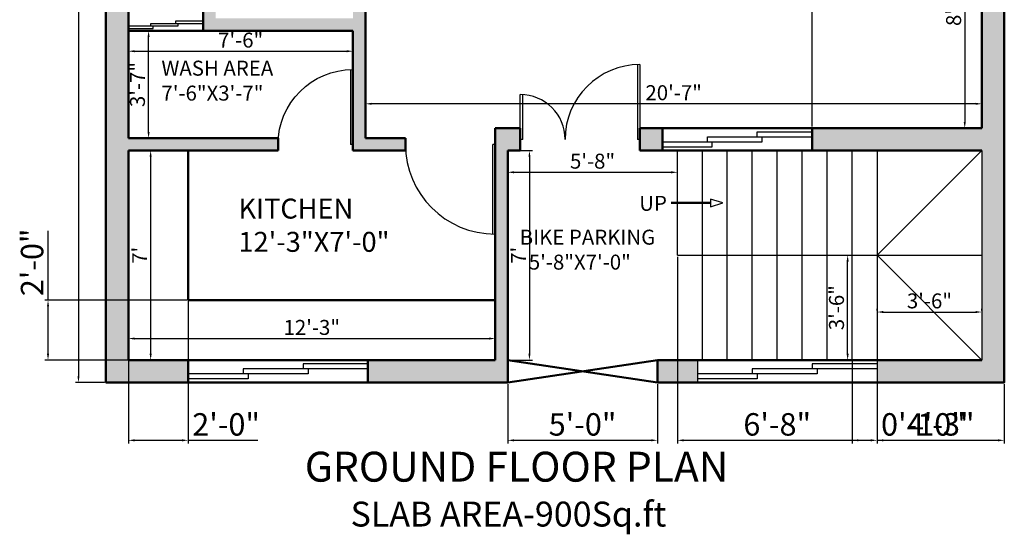
# Model space of a CAD drawing. Units: inches. Extents: x 3274 to 5176, y 1085 to 2172.
# Tile 1 of 16: x 3339 to 3733, y 1118 to 1325. Entities that reach past the tile are written whole.
import ezdxf

# ---------------------------------------------------------------- set-up
doc = ezdxf.new("R2010")
doc.units = ezdxf.units.IN
for name, color, linetype, lineweight in [('A-ANNO-DIMS', 2, 'Continuous', 18), ('A-ANNO-TEXT', 7, 'Continuous', 25), ('A-AREA-IDEN', 3, 'Continuous', 25), ('A-DOOR', 4, 'Continuous', 25), ('A-FLOR-STRS', 7, 'Continuous', 25), ('A-GLAZ', 5, 'Continuous', 25), ('A-WALL', 7, 'Continuous', 50), ('A-WALL-PATT', 8, 'Continuous', 13)]:
    doc.layers.add(name, color=color, linetype=linetype, lineweight=lineweight)
doc.styles.get("Standard").update_dxf_attribs({"font": 'arial.ttf'})
doc.dimstyles.new('ISO-25', dxfattribs={"dimtxt": 9, "dimasz": 2.5, "dimexe": 1.25, "dimexo": 0.625, "dimtad": 1, "dimdec": 1, "dimlunit": 3, "dimtxsty": 'Standard', "dimcen": 2.5, "dimclrd": 4, "dimclre": 4, "dimclrt": 1, "dimadec": 0, "dimazin": 0, "dimtfac": 1, "dimtdec": 1, "dimtmove": 0, "dimatfit": 3, "dimfxl": 1, "dimarcsym": 0})

# ---------------------------------------------------------------- blocks, each defined once
blk = doc.blocks.new('3')
for p, q in [((47, 30), (47, 0)), ((48, 30), (48, 0)), ((0, 0), (0, 18)), ((1, 0), (1, 18)), ((1, 0), (0, 0)), ((48, 0), (47, 0))]:
    blk.add_line(p, q)
for centre, radius, start, end in [((48, 0), 30, 90, 180), ((0, 0), 18, 0, 90)]:
    blk.add_arc(centre, radius, start, end)
blk = doc.blocks.new('2')
for p, q in [((0, 30), (0, 0)), ((1, 30), (1, 0)), ((0, 0), (1, 0))]:
    blk.add_line(p, q)
blk.add_arc((0, 0), 30, 0, 90)
blk = doc.blocks.new('1')
for p, q in [((0, 36), (0, 0)), ((1, 36), (1, 0)), ((0, 0), (1, 0))]:
    blk.add_line(p, q)
blk.add_arc((0, 0), 36, 0, 90)
blk = doc.blocks.new('*D11')
at = {"layer": 'A-ANNO-DIMS', "color": 0, "lineweight": -2, "transparency": 16777216}
for p, q in [((3372.68, 1539.28), (3361.05, 1539.28)), ((3362.3, 1536.78), (3362.3, 1181.78)), ((3372.68, 1179.28), (3361.05, 1179.28))]:
    blk.add_line(p, q, dxfattribs=at)
at = {"layer": 'A-ANNO-DIMS', "color": 0, "transparency": 16777216}
for points in [[(3361.88, 1536.78), (3362.71, 1536.78), (3362.3, 1539.28)], [(3361.88, 1181.78), (3362.71, 1181.78), (3362.3, 1179.28)]]:
    blk.add_solid(points, dxfattribs=at)
at = {"layer": 'Defpoints', "color": 0, "transparency": 16777216}
for p in [(3373.3, 1539.28), (3362.3, 1179.28), (3373.3, 1179.28)]:
    blk.add_point(p, dxfattribs=at)
at = {"layer": 'A-ANNO-DIMS', "color": 0, "transparency": 16777216, "insert": (3357.07, 1359.28), "char_height": 9, "attachment_point": 5, "rotation": 90}
blk.add_mtext("30'", dxfattribs=at)
blk = doc.blocks.new('*D20')
at = {"layer": 'A-ANNO-DIMS', "color": 0, "lineweight": -2, "transparency": 16777216}
for p, q in [((3382.93, 1320.28), (3391.65, 1320.28)), ((3390.4, 1279.78), (3390.4, 1317.78)), ((3382.93, 1277.28), (3391.65, 1277.28))]:
    blk.add_line(p, q, dxfattribs=at)
at = {"layer": 'A-ANNO-DIMS', "color": 0, "transparency": 16777216}
for points in [[(3389.98, 1317.78), (3390.82, 1317.78), (3390.4, 1320.28)], [(3389.98, 1279.78), (3390.82, 1279.78), (3390.4, 1277.28)]]:
    blk.add_solid(points, dxfattribs=at)
at = {"layer": 'Defpoints', "color": 0, "transparency": 16777216}
for p in [(3382.3, 1320.28), (3390.4, 1320.28), (3382.3, 1277.28)]:
    blk.add_point(p, dxfattribs=at)
at = {"layer": 'A-ANNO-DIMS', "color": 0, "transparency": 16777216, "insert": (3386.71, 1298.78), "char_height": 6, "attachment_point": 5, "rotation": 90}
blk.add_mtext('3\'-7"', dxfattribs=at)
blk = doc.blocks.new('*D21')
at = {"layer": 'A-ANNO-DIMS', "color": 0, "lineweight": -2, "transparency": 16777216}
for p, q in [((3382.3, 1319.66), (3382.3, 1310.87)), ((3472.3, 1319.66), (3472.3, 1310.87)), ((3384.8, 1312.12), (3469.8, 1312.12))]:
    blk.add_line(p, q, dxfattribs=at)
at = {"layer": 'A-ANNO-DIMS', "color": 0, "transparency": 16777216}
for points in [[(3384.8, 1312.54), (3384.8, 1311.7), (3382.3, 1312.12)], [(3469.8, 1312.54), (3469.8, 1311.7), (3472.3, 1312.12)]]:
    blk.add_solid(points, dxfattribs=at)
at = {"layer": 'Defpoints', "color": 0, "transparency": 16777216}
for p in [(3382.3, 1320.28), (3472.3, 1320.28), (3472.3, 1312.12)]:
    blk.add_point(p, dxfattribs=at)
at = {"layer": 'A-ANNO-DIMS', "color": 0, "transparency": 16777216, "insert": (3427.3, 1315.81), "char_height": 6, "attachment_point": 5}
blk.add_mtext('7\'-6"', dxfattribs=at)
blk = doc.blocks.new('*D22')
at = {"layer": 'A-ANNO-DIMS', "color": 0, "lineweight": -2, "transparency": 16777216}
for p, q in [((3382.93, 1272.28), (3392.47, 1272.28)), ((3391.22, 1269.78), (3391.22, 1190.78)), ((3382.93, 1188.28), (3392.47, 1188.28))]:
    blk.add_line(p, q, dxfattribs=at)
at = {"layer": 'A-ANNO-DIMS', "color": 0, "transparency": 16777216}
for points in [[(3390.81, 1269.78), (3391.64, 1269.78), (3391.22, 1272.28)], [(3390.81, 1190.78), (3391.64, 1190.78), (3391.22, 1188.28)]]:
    blk.add_solid(points, dxfattribs=at)
at = {"layer": 'Defpoints', "color": 0, "transparency": 16777216}
for p in [(3382.3, 1272.28), (3382.3, 1188.28), (3391.22, 1188.28)]:
    blk.add_point(p, dxfattribs=at)
at = {"layer": 'A-ANNO-DIMS', "color": 0, "transparency": 16777216, "insert": (3387.6, 1230.28), "char_height": 6, "attachment_point": 5, "rotation": 90}
blk.add_mtext("7'", dxfattribs=at)
blk = doc.blocks.new('*D23')
at = {"layer": 'A-ANNO-DIMS', "color": 0, "lineweight": -2, "transparency": 16777216}
for p, q in [((3382.3, 1188.91), (3382.3, 1198.14)), ((3384.8, 1196.89), (3526.8, 1196.89)), ((3529.3, 1188.91), (3529.3, 1198.14))]:
    blk.add_line(p, q, dxfattribs=at)
at = {"layer": 'A-ANNO-DIMS', "color": 0, "transparency": 16777216}
for points in [[(3384.8, 1197.31), (3384.8, 1196.47), (3382.3, 1196.89)], [(3526.8, 1197.31), (3526.8, 1196.47), (3529.3, 1196.89)]]:
    blk.add_solid(points, dxfattribs=at)
at = {"layer": 'Defpoints', "color": 0, "transparency": 16777216}
for p in [(3529.3, 1196.89), (3382.3, 1188.28), (3529.3, 1188.28)]:
    blk.add_point(p, dxfattribs=at)
at = {"layer": 'A-ANNO-DIMS', "color": 0, "transparency": 16777216, "insert": (3455.8, 1200.58), "char_height": 6, "attachment_point": 5}
blk.add_mtext('12\'-3"', dxfattribs=at)
blk = doc.blocks.new('*D24')
at = {"layer": 'A-ANNO-DIMS', "color": 0, "lineweight": -2, "transparency": 16777216}
for p, q in [((3534.3, 1262.94), (3534.3, 1262.32)), ((3536.8, 1263.57), (3599.8, 1263.57)), ((3602.3, 1264.19), (3602.3, 1264.82))]:
    blk.add_line(p, q, dxfattribs=at)
at = {"layer": 'A-ANNO-DIMS', "color": 0, "transparency": 16777216}
for points in [[(3536.8, 1263.99), (3536.8, 1263.15), (3534.3, 1263.57)], [(3599.8, 1263.99), (3599.8, 1263.15), (3602.3, 1263.57)]]:
    blk.add_solid(points, dxfattribs=at)
at = {"layer": 'Defpoints', "color": 0, "transparency": 16777216}
for p in [(3534.3, 1263.57), (3602.3, 1263.57), (3602.3, 1263.57)]:
    blk.add_point(p, dxfattribs=at)
at = {"layer": 'A-ANNO-DIMS', "color": 0, "transparency": 16777216, "insert": (3568.3, 1267.26), "char_height": 6, "attachment_point": 5}
blk.add_mtext('5\'-8"', dxfattribs=at)
blk = doc.blocks.new('*D25')
at = {"layer": 'A-ANNO-DIMS', "color": 0, "lineweight": -2, "transparency": 16777216}
for p, q in [((3534.93, 1272.28), (3544.26, 1272.28)), ((3543.01, 1269.78), (3543.01, 1190.78)), ((3534.93, 1188.28), (3544.26, 1188.28))]:
    blk.add_line(p, q, dxfattribs=at)
at = {"layer": 'A-ANNO-DIMS', "color": 0, "transparency": 16777216}
for points in [[(3542.6, 1269.78), (3543.43, 1269.78), (3543.01, 1272.28)], [(3542.6, 1190.78), (3543.43, 1190.78), (3543.01, 1188.28)]]:
    blk.add_solid(points, dxfattribs=at)
at = {"layer": 'Defpoints', "color": 0, "transparency": 16777216}
for p in [(3534.3, 1272.28), (3534.3, 1188.28), (3543.01, 1188.28)]:
    blk.add_point(p, dxfattribs=at)
at = {"layer": 'A-ANNO-DIMS', "color": 0, "transparency": 16777216, "insert": (3539.39, 1230.28), "char_height": 6, "attachment_point": 5, "rotation": 90}
blk.add_mtext("7'", dxfattribs=at)
blk = doc.blocks.new('*D26')
at = {"layer": 'A-ANNO-DIMS', "color": 0, "lineweight": -2, "transparency": 16777216}
for p, q in [((3668.38, 1230.28), (3671.77, 1230.28)), ((3670.52, 1190.78), (3670.52, 1227.78)), ((3668.38, 1188.28), (3671.77, 1188.28))]:
    blk.add_line(p, q, dxfattribs=at)
at = {"layer": 'A-ANNO-DIMS', "color": 0, "transparency": 16777216}
for points in [[(3670.1, 1227.78), (3670.94, 1227.78), (3670.52, 1230.28)], [(3670.1, 1190.78), (3670.94, 1190.78), (3670.52, 1188.28)]]:
    blk.add_solid(points, dxfattribs=at)
at = {"layer": 'Defpoints', "color": 0, "transparency": 16777216}
for p in [(3667.75, 1230.28), (3670.52, 1230.28), (3667.75, 1188.28)]:
    blk.add_point(p, dxfattribs=at)
at = {"layer": 'A-ANNO-DIMS', "color": 0, "transparency": 16777216, "insert": (3666.83, 1209.28), "char_height": 6, "attachment_point": 5, "rotation": 90}
blk.add_mtext('3\'-6"', dxfattribs=at)
blk = doc.blocks.new('*D27')
at = {"layer": 'A-ANNO-DIMS', "color": 0, "lineweight": -2, "transparency": 16777216}
for p, q in [((3682.3, 1208.15), (3682.3, 1208.78)), ((3684.8, 1207.53), (3721.8, 1207.53)), ((3724.3, 1208.15), (3724.3, 1208.78))]:
    blk.add_line(p, q, dxfattribs=at)
at = {"layer": 'A-ANNO-DIMS', "color": 0, "transparency": 16777216}
for points in [[(3684.8, 1207.95), (3684.8, 1207.11), (3682.3, 1207.53)], [(3721.8, 1207.95), (3721.8, 1207.11), (3724.3, 1207.53)]]:
    blk.add_solid(points, dxfattribs=at)
at = {"layer": 'Defpoints', "color": 0, "transparency": 16777216}
for p in [(3682.3, 1207.53), (3724.3, 1207.53), (3724.3, 1207.53)]:
    blk.add_point(p, dxfattribs=at)
at = {"layer": 'A-ANNO-DIMS', "color": 0, "transparency": 16777216, "insert": (3703.3, 1211.22), "char_height": 6, "attachment_point": 5}
blk.add_mtext('3\'-6"', dxfattribs=at)
blk = doc.blocks.new('*D28')
at = {"layer": 'A-ANNO-DIMS', "color": 0, "lineweight": -2, "transparency": 16777216}
for p, q in [((3723.68, 1381.28), (3716.2, 1381.28)), ((3717.45, 1378.78), (3717.45, 1283.78)), ((3723.68, 1281.28), (3716.2, 1281.28))]:
    blk.add_line(p, q, dxfattribs=at)
at = {"layer": 'A-ANNO-DIMS', "color": 0, "transparency": 16777216}
for points in [[(3717.03, 1378.78), (3717.86, 1378.78), (3717.45, 1381.28)], [(3717.03, 1283.78), (3717.86, 1283.78), (3717.45, 1281.28)]]:
    blk.add_solid(points, dxfattribs=at)
at = {"layer": 'Defpoints', "color": 0, "transparency": 16777216}
for p in [(3724.3, 1381.28), (3717.45, 1281.28), (3724.3, 1281.28)]:
    blk.add_point(p, dxfattribs=at)
at = {"layer": 'A-ANNO-DIMS', "color": 0, "transparency": 16777216, "insert": (3713.76, 1331.28), "char_height": 6, "attachment_point": 5, "rotation": 90}
blk.add_mtext('8\'-4"', dxfattribs=at)
blk = doc.blocks.new('*D29')
at = {"layer": 'A-ANNO-DIMS', "color": 0, "lineweight": -2, "transparency": 16777216}
for p, q in [((3477.3, 1277.91), (3477.3, 1292.29)), ((3721.8, 1291.04), (3479.8, 1291.04)), ((3724.3, 1281.91), (3724.3, 1292.29))]:
    blk.add_line(p, q, dxfattribs=at)
at = {"layer": 'A-ANNO-DIMS', "color": 0, "transparency": 16777216}
for points in [[(3479.8, 1291.45), (3479.8, 1290.62), (3477.3, 1291.04)], [(3721.8, 1291.45), (3721.8, 1290.62), (3724.3, 1291.04)]]:
    blk.add_solid(points, dxfattribs=at)
at = {"layer": 'Defpoints', "color": 0, "transparency": 16777216}
for p in [(3477.3, 1291.04), (3724.3, 1281.28), (3477.3, 1277.28)]:
    blk.add_point(p, dxfattribs=at)
at = {"layer": 'A-ANNO-DIMS', "color": 0, "transparency": 16777216, "insert": (3600.8, 1294.72), "char_height": 6, "attachment_point": 5}
blk.add_mtext('20\'-7"', dxfattribs=at)
blk = doc.blocks.new('WIN-30')
for p, q in [((4385.19, 1318.35), (4396.19, 1318.35)), ((4385.19, 1317.35), (4385.19, 1318.35)), ((4366.19, 1316.35), (4386.19, 1316.35)), ((4366.19, 1315.35), (4376.19, 1315.35)), ((4375.19, 1317.35), (4396.19, 1317.35)), ((4375.19, 1316.35), (4375.19, 1317.35)), ((4376.19, 1315.35), (4376.19, 1316.35)), ((4386.19, 1316.35), (4386.19, 1317.35))]:
    blk.add_line(p, q)
blk = doc.blocks.new('WIN-60')
for p, q in [((4598.19, 1271.85), (4640.19, 1271.85)), ((4598.19, 1269.85), (4598.19, 1271.85)), ((4618.19, 1273.85), (4640.19, 1273.85)), ((4618.19, 1271.85), (4618.19, 1273.85)), ((4620.19, 1269.85), (4620.19, 1271.85)), ((4580.19, 1269.85), (4620.19, 1269.85)), ((4580.19, 1267.85), (4600.19, 1267.85)), ((4600.19, 1267.85), (4600.19, 1269.85))]:
    blk.add_line(p, q)
blk = doc.blocks.new('WIN-72')
for p, q in [((4462.19, 1180.85), (4436.19, 1180.85)), ((4436.19, 1180.85), (4436.19, 1178.85)), ((4438.19, 1176.85), (4390.19, 1176.85)), ((4462.19, 1178.85), (4412.19, 1178.85)), ((4412.19, 1178.85), (4412.19, 1176.85)), ((4414.19, 1176.85), (4414.19, 1174.85)), ((4438.19, 1178.85), (4438.19, 1176.85)), ((4414.19, 1174.85), (4390.19, 1174.85))]:
    blk.add_line(p, q)
blk = doc.blocks.new('*D160')
at = {"layer": 'A-ANNO-DIMS', "color": 4, "lineweight": -2, "transparency": 16777216}
for p, q in [((3682.3, 1178.66), (3682.3, 1154.83)), ((3733.3, 1178.66), (3733.3, 1154.83)), ((3684.8, 1156.08), (3730.8, 1156.08))]:
    blk.add_line(p, q, dxfattribs=at)
at = {"layer": 'A-ANNO-DIMS', "color": 4, "transparency": 16777216}
for points in [[(3684.8, 1156.5), (3684.8, 1155.66), (3682.3, 1156.08)], [(3730.8, 1156.5), (3730.8, 1155.66), (3733.3, 1156.08)]]:
    blk.add_solid(points, dxfattribs=at)
at = {"layer": 'Defpoints', "color": 0, "transparency": 16777216}
for p in [(3682.3, 1179.28), (3733.3, 1179.28), (3733.3, 1156.08)]:
    blk.add_point(p, dxfattribs=at)
at = {"layer": 'A-ANNO-DIMS', "color": 1, "transparency": 16777216, "insert": (3707.8, 1161.3), "char_height": 9, "attachment_point": 5}
blk.add_mtext('4\'-3"', dxfattribs=at)
blk = doc.blocks.new('*D161')
at = {"layer": 'A-ANNO-DIMS', "color": 4, "lineweight": -2, "transparency": 16777216}
for p, q in [((3534.3, 1178.66), (3534.3, 1154.83)), ((3594.3, 1178.66), (3594.3, 1154.83)), ((3536.8, 1156.08), (3591.8, 1156.08))]:
    blk.add_line(p, q, dxfattribs=at)
at = {"layer": 'A-ANNO-DIMS', "color": 4, "transparency": 16777216}
for points in [[(3536.8, 1156.5), (3536.8, 1155.66), (3534.3, 1156.08)], [(3591.8, 1156.5), (3591.8, 1155.66), (3594.3, 1156.08)]]:
    blk.add_solid(points, dxfattribs=at)
at = {"layer": 'Defpoints', "color": 0, "transparency": 16777216}
for p in [(3534.3, 1179.28), (3594.3, 1179.28), (3594.3, 1156.08)]:
    blk.add_point(p, dxfattribs=at)
at = {"layer": 'A-ANNO-DIMS', "color": 1, "transparency": 16777216, "insert": (3564.3, 1161.3), "char_height": 9, "attachment_point": 5}
blk.add_mtext('5\'-0"', dxfattribs=at)
blk = doc.blocks.new('*D162')
at = {"layer": 'A-ANNO-DIMS', "color": 4, "lineweight": -2, "transparency": 16777216}
for p, q in [((3382.3, 1271.66), (3382.3, 1154.83)), ((3406.3, 1271.66), (3406.3, 1154.83)), ((3384.8, 1156.08), (3403.8, 1156.08)), ((3406.3, 1156.08), (3434.13, 1156.08))]:
    blk.add_line(p, q, dxfattribs=at)
at = {"layer": 'A-ANNO-DIMS', "color": 4, "transparency": 16777216}
for points in [[(3384.8, 1156.5), (3384.8, 1155.66), (3382.3, 1156.08)], [(3403.8, 1156.5), (3403.8, 1155.66), (3406.3, 1156.08)]]:
    blk.add_solid(points, dxfattribs=at)
at = {"layer": 'Defpoints', "color": 0, "transparency": 16777216}
for p in [(3382.3, 1272.28), (3406.3, 1272.28), (3406.3, 1156.08)]:
    blk.add_point(p, dxfattribs=at)
at = {"layer": 'A-ANNO-DIMS', "color": 1, "transparency": 16777216, "insert": (3421.46, 1161.3), "char_height": 9, "attachment_point": 5}
blk.add_mtext('2\'-0"', dxfattribs=at)
blk = doc.blocks.new('*D163')
at = {"layer": 'A-ANNO-DIMS', "color": 4, "lineweight": -2, "transparency": 16777216}
for p, q in [((3350.1, 1212.28), (3350.1, 1240.11)), ((3405.68, 1212.28), (3348.85, 1212.28)), ((3350.1, 1190.78), (3350.1, 1209.78)), ((3405.68, 1188.28), (3348.85, 1188.28))]:
    blk.add_line(p, q, dxfattribs=at)
at = {"layer": 'A-ANNO-DIMS', "color": 4, "transparency": 16777216}
for points in [[(3349.68, 1209.78), (3350.52, 1209.78), (3350.1, 1212.28)], [(3349.68, 1190.78), (3350.52, 1190.78), (3350.1, 1188.28)]]:
    blk.add_solid(points, dxfattribs=at)
at = {"layer": 'Defpoints', "color": 0, "transparency": 16777216}
for p in [(3350.1, 1212.28), (3406.3, 1212.28), (3406.3, 1188.28)]:
    blk.add_point(p, dxfattribs=at)
at = {"layer": 'A-ANNO-DIMS', "color": 1, "transparency": 16777216, "insert": (3344.88, 1227.45), "char_height": 9, "attachment_point": 5, "rotation": 90}
blk.add_mtext('2\'-0"', dxfattribs=at)
blk = doc.blocks.new('*D164')
at = {"layer": 'A-ANNO-DIMS', "color": 4, "lineweight": -2, "transparency": 16777216}
for p, q in [((3602.3, 1229.66), (3602.3, 1154.83)), ((3682.3, 1229.66), (3682.3, 1154.83)), ((3604.8, 1156.08), (3679.8, 1156.08))]:
    blk.add_line(p, q, dxfattribs=at)
at = {"layer": 'A-ANNO-DIMS', "color": 4, "transparency": 16777216}
for points in [[(3604.8, 1156.5), (3604.8, 1155.66), (3602.3, 1156.08)], [(3679.8, 1156.5), (3679.8, 1155.66), (3682.3, 1156.08)]]:
    blk.add_solid(points, dxfattribs=at)
at = {"layer": 'Defpoints', "color": 0, "transparency": 16777216}
for p in [(3602.3, 1230.28), (3682.3, 1230.28), (3682.3, 1156.08)]:
    blk.add_point(p, dxfattribs=at)
at = {"layer": 'A-ANNO-DIMS', "color": 1, "transparency": 16777216, "insert": (3642.3, 1161.3), "char_height": 9, "attachment_point": 5}
blk.add_mtext('6\'-8"', dxfattribs=at)
blk = doc.blocks.new('*D165')
at = {"layer": 'A-ANNO-DIMS', "color": 4, "lineweight": -2, "transparency": 16777216}
for p, q in [((3672.3, 1187.66), (3672.3, 1154.83)), ((3682.3, 1187.66), (3682.3, 1154.83)), ((3674.8, 1156.08), (3679.8, 1156.08)), ((3682.3, 1156.08), (3716.97, 1156.08))]:
    blk.add_line(p, q, dxfattribs=at)
at = {"layer": 'A-ANNO-DIMS', "color": 4, "transparency": 16777216}
for points in [[(3674.8, 1156.5), (3674.8, 1155.66), (3672.3, 1156.08)], [(3679.8, 1156.5), (3679.8, 1155.66), (3682.3, 1156.08)]]:
    blk.add_solid(points, dxfattribs=at)
at = {"layer": 'Defpoints', "color": 0, "transparency": 16777216}
for p in [(3672.3, 1188.28), (3682.3, 1188.28), (3682.3, 1156.08)]:
    blk.add_point(p, dxfattribs=at)
at = {"layer": 'A-ANNO-DIMS', "color": 1, "transparency": 16777216, "insert": (3700.88, 1161.3), "char_height": 9, "attachment_point": 5}
blk.add_mtext('0\'-10"', dxfattribs=at)
blk = doc.blocks.new('*D166')
at = {"layer": 'A-ANNO-DIMS', "color": 4, "lineweight": -2, "transparency": 16777216}
for p, q in [((3656.3, 1281.91), (3656.3, 1563.73)), ((3658.8, 1562.48), (3721.8, 1562.48)), ((3724.3, 1281.91), (3724.3, 1563.73))]:
    blk.add_line(p, q, dxfattribs=at)
at = {"layer": 'A-ANNO-DIMS', "color": 4, "transparency": 16777216}
for points in [[(3658.8, 1562.9), (3658.8, 1562.06), (3656.3, 1562.48)], [(3721.8, 1562.9), (3721.8, 1562.06), (3724.3, 1562.48)]]:
    blk.add_solid(points, dxfattribs=at)
at = {"layer": 'Defpoints', "color": 0, "transparency": 16777216}
for p in [(3724.3, 1562.48), (3656.3, 1281.28), (3724.3, 1281.28)]:
    blk.add_point(p, dxfattribs=at)
at = {"layer": 'A-ANNO-DIMS', "color": 1, "transparency": 16777216, "insert": (3690.3, 1567.7), "char_height": 9, "attachment_point": 5}
blk.add_mtext('5\'-8"', dxfattribs=at)

msp = doc.modelspace()

# ---------------------------------------------------------------- hatches: boundary and pattern name
at = {"layer": 'A-WALL-PATT'}
h = msp.add_hatch(color=256, dxfattribs=at)
h.dxf.hatch_style = 1
h.paths.add_polyline_path([(3733.3, 1539.28), (3373.3, 1539.28), (3373.3, 1179.28), (3406.3, 1179.28), (3406.3, 1188.28), (3382.3, 1188.28), (3382.3, 1272.28), (3442.3, 1272.28), (3442.3, 1277.28), (3382.3, 1277.28), (3382.3, 1381.28), (3442.3, 1381.28), (3442.3, 1386.28), (3382.3, 1386.28), (3382.3, 1530.28), (3724.3, 1530.28), (3724.3, 1386.28), (3594.3, 1386.28), (3594.3, 1381.28), (3724.3, 1381.28), (3724.3, 1281.28), (3656.3, 1281.28), (3656.3, 1272.28), (3724.3, 1272.28), (3724.3, 1188.28), (3682.3, 1188.28), (3682.3, 1179.28), (3733.3, 1179.28)])
h.paths.add_polyline_path([(3477.3, 1381.28), (3493.3, 1381.28), (3493.3, 1386.28), (3472.3, 1386.28), (3472.3, 1325.28), (3417.3, 1325.28), (3417.3, 1345.28), (3412.3, 1345.28), (3412.3, 1320.28), (3472.3, 1320.28), (3472.3, 1272.28), (3493.3, 1272.28), (3493.3, 1277.28), (3477.3, 1277.28)], flags=17)
h.paths.add_polyline_path([(3534.3, 1489.28), (3552.3, 1489.28), (3552.3, 1494.28), (3529.3, 1494.28), (3529.3, 1381.28), (3552.3, 1381.28), (3552.3, 1386.28), (3534.3, 1386.28), (3534.3, 1424.28), (3564.3, 1424.28), (3564.3, 1429.28), (3534.3, 1429.28)], flags=17)
h.paths.add_polyline_path([(3599.3, 1494.28), (3576.3, 1494.28), (3576.3, 1489.28), (3594.3, 1489.28), (3594.3, 1422.28), (3599.3, 1422.28)], flags=17)
h.paths.add_polyline_path([(3534.3, 1272.28), (3539.3, 1272.28), (3539.3, 1281.28), (3529.3, 1281.28), (3529.3, 1188.28), (3478.3, 1188.28), (3478.3, 1179.28), (3534.3, 1179.28)], flags=17)
h.paths.add_polyline_path([(3596.3, 1281.28), (3587.3, 1281.28), (3587.3, 1276.78), (3587.3, 1272.28), (3596.3, 1272.28)], flags=17)
h.paths.add_polyline_path([(3610.3, 1188.28), (3594.3, 1188.28), (3594.3, 1179.28), (3610.3, 1179.28)], flags=17)
h.paths.add_polyline_path([(3589.35, 1322.21), (3663.55, 1322.21), (3663.55, 1352.06), (3589.35, 1352.06)], flags=25)
h.paths.add_polyline_path([(3545.54, 1458.93), (3584.72, 1458.93), (3584.72, 1481.32), (3545.54, 1481.32)], flags=25)
h.paths.add_polyline_path([(3635.11, 1449.68), (3703.51, 1449.68), (3703.51, 1479.54), (3635.11, 1479.54)], flags=25)
h.paths.add_polyline_path([(3543.78, 1502.97), (3585.75, 1502.97), (3585.75, 1525.36), (3543.78, 1525.36)], flags=25)
h.paths.add_polyline_path([(3423.19, 1449.68), (3491.58, 1449.68), (3491.58, 1479.54), (3423.19, 1479.54)], flags=25)

# ---------------------------------------------------------------- linework, layer by layer
at = {"layer": 'A-FLOR-STRS'}
for p, q in [((3602.3, 1230.28), (3602.3, 1272.28)), ((3612.3, 1230.28), (3612.3, 1272.28)), ((3622.3, 1230.28), (3622.3, 1272.28)), ((3632.3, 1230.28), (3632.3, 1272.28)), ((3642.3, 1230.28), (3642.3, 1272.28)), ((3652.3, 1230.28), (3652.3, 1272.28)), ((3662.3, 1230.28), (3662.3, 1272.28)), ((3672.3, 1230.28), (3672.3, 1272.28)), ((3682.3, 1272.28), (3682.3, 1188.28)), ((3682.3, 1230.28), (3724.3, 1272.28)), ((3724.3, 1272.28), (3724.3, 1188.28)), ((3602.3, 1230.28), (3724.3, 1230.28)), ((3612.3, 1188.28), (3612.3, 1230.28)), ((3622.3, 1188.28), (3622.3, 1230.28)), ((3632.3, 1188.28), (3632.3, 1230.28)), ((3642.3, 1188.28), (3642.3, 1230.28)), ((3652.3, 1188.28), (3652.3, 1230.28)), ((3662.3, 1188.28), (3662.3, 1230.28)), ((3672.3, 1188.28), (3672.3, 1230.28)), ((3682.3, 1230.28), (3724.3, 1188.28)), ((3610.3, 1188.28), (3610.3, 1179.28)), ((3682.3, 1188.28), (3682.3, 1179.28))]:
    msp.add_line(p, q, dxfattribs=at)
msp.add_lwpolyline([(3620.5, 1251.28), (3615.62, 1252.78), (3615.62, 1249.78)], close=True, dxfattribs=at)
at = {"layer": 'A-WALL'}
for p, q in [((3382.3, 1277.28), (3382.3, 1381.28)), ((3477.3, 1277.28), (3477.3, 1381.28)), ((3724.3, 1381.28), (3724.3, 1281.28)), ((3412.3, 1320.28), (3412.3, 1345.28)), ((3382.3, 1320.28), (3472.3, 1320.28)), ((3472.3, 1272.28), (3472.3, 1320.28)), ((3529.3, 1281.28), (3539.3, 1281.28)), ((3529.3, 1188.28), (3529.3, 1281.28)), ((3539.3, 1272.28), (3539.3, 1281.28)), ((3587.3, 1281.28), (3724.3, 1281.28)), ((3587.3, 1272.28), (3587.3, 1281.28)), ((3596.3, 1272.28), (3596.3, 1281.28)), ((3656.3, 1272.28), (3656.3, 1281.28)), ((3382.3, 1277.28), (3442.3, 1277.28)), ((3442.3, 1272.28), (3442.3, 1277.28)), ((3477.3, 1277.28), (3493.3, 1277.28)), ((3493.3, 1272.28), (3493.3, 1277.28)), ((3382.3, 1272.28), (3442.3, 1272.28)), ((3382.3, 1188.28), (3382.3, 1272.28)), ((3406.3, 1212.28), (3406.3, 1272.28)), ((3472.3, 1272.28), (3493.3, 1272.28)), ((3534.3, 1272.28), (3539.3, 1272.28)), ((3534.3, 1179.28), (3534.3, 1272.28)), ((3587.3, 1272.28), (3724.3, 1272.28)), ((3599.86, 1251.28), (3615.62, 1251.28)), ((3529.3, 1212.28), (3406.3, 1212.28)), ((3529.3, 1188.28), (3382.3, 1188.28)), ((3406.3, 1188.28), (3406.3, 1179.28)), ((3478.3, 1188.28), (3478.3, 1179.28)), ((3534.3, 1179.28), (3594.3, 1188.28)), ((3594.3, 1179.28), (3534.3, 1188.28)), ((3724.3, 1188.28), (3594.3, 1188.28)), ((3594.3, 1179.28), (3594.3, 1188.28))]:
    msp.add_line(p, q, dxfattribs=at)
msp.add_lwpolyline([(3534.3, 1179.28), (3373.3, 1179.28), (3373.3, 1539.28), (3733.3, 1539.28), (3733.3, 1179.28), (3594.3, 1179.28)], dxfattribs=at)

# ---------------------------------------------------------------- block references
at = {"layer": 'A-DOOR'}
msp.add_blockref('3', (3539.3, 1276.78), dxfattribs=at)
at = {"layer": 'A-DOOR', "xscale": -1}
msp.add_blockref('2', (3472.3, 1274.78), dxfattribs=at)
at = {"layer": 'A-DOOR', "rotation": 180}
msp.add_blockref('1', (3529.3, 1274.78), dxfattribs=at)
at = {"layer": 'A-GLAZ'}
for name, p in [('WIN-30', (-983.89, 5.93)), ('WIN-60', (-983.89, 5.93)), ('WIN-72', (-983.89, 5.93)), ('WIN-72', (-779.89, 5.93))]:
    msp.add_blockref(name, p, dxfattribs=at)

# ---------------------------------------------------------------- texts
at = {"layer": 'A-ANNO-TEXT'}
msp.add_text('UP', height=6, dxfattribs=at).set_placement((3587.01, 1248.13))
at = {"layer": 'A-ANNO-TEXT', "insert": (3452.99, 1151.5), "char_height": 12, "attachment_point": 1}
msp.add_mtext_dynamic_manual_height_columns('GROUND FLOOR PLAN\\P{\\H0.83333x;      SLAB AREA-900Sq.ft}', width=202.3193, gutter_width=30, heights=[0], dxfattribs=at)
at = {"layer": 'A-AREA-IDEN', "attachment_point": 1}
for s, insert, char_height in [('WASH AREA\\P7\'-6"X3\'-7"', (3395.55, 1308.33), 6), ('KITCHEN\\P12\'-3"X7\'-0"', (3426.41, 1253.01), 8), ('BIKE PARKING\\P  5\'-8"X7\'-0"', (3539.11, 1240.55), 6)]:
    msp.add_mtext_dynamic_manual_height_columns(s, width=58.0121, gutter_width=30, heights=[0], dxfattribs=dict(at, insert=insert, char_height=char_height))

# ---------------------------------------------------------------- dimensions: what is measured, and where the dimension line sits
at = {"layer": 'A-ANNO-DIMS'}
for base, p1, p2, override, picture, middle in [((3724.3, 1562.48), (3656.3, 1281.28), (3724.3, 1281.28), {"dimdec": 1, "dimlfac": 1, "dimrnd": 0, "dimzin": 1, "dimdsep": 46, "dimlunit": 4, "dimfrac": 2}, '*D166', (3690.3, 1567.7)), ((3472.3, 1312.12), (3382.3, 1320.28), (3472.3, 1320.28), {"dimtxt": 6, "dimclrd": 0, "dimclre": 0, "dimclrt": 0}, '*D21', (3427.3, 1315.81)), ((3477.3, 1291.04), (3724.3, 1281.28), (3477.3, 1277.28), {"dimtxt": 6, "dimclrd": 0, "dimclre": 0, "dimclrt": 0}, '*D29', (3600.8, 1294.72)), ((3406.3, 1156.08), (3382.3, 1272.28), (3406.3, 1272.28), {"dimdec": 1, "dimlfac": 1, "dimrnd": 0, "dimzin": 1, "dimdsep": 46, "dimlunit": 4, "dimfrac": 2}, '*D162', (3421.46, 1161.3)), ((3602.3, 1263.57), (3534.3, 1263.57), (3602.3, 1263.57), {"dimtxt": 6, "dimclrd": 0, "dimclre": 0, "dimclrt": 0}, '*D24', (3568.3, 1267.26)), ((3682.3, 1156.08), (3602.3, 1230.28), (3682.3, 1230.28), {"dimdec": 1, "dimlfac": 1, "dimrnd": 0, "dimzin": 1, "dimdsep": 46, "dimlunit": 4, "dimfrac": 2}, '*D164', (3642.3, 1161.3)), ((3724.3, 1207.53), (3682.3, 1207.53), (3724.3, 1207.53), {"dimtxt": 6, "dimclrd": 0, "dimclre": 0, "dimclrt": 0}, '*D27', (3703.3, 1211.22)), ((3529.3, 1196.89), (3382.3, 1188.28), (3529.3, 1188.28), {"dimtxt": 6, "dimclrd": 0, "dimclre": 0, "dimclrt": 0}, '*D23', (3455.8, 1200.58)), ((3682.3, 1156.08), (3672.3, 1188.28), (3682.3, 1188.28), {"dimdec": 1, "dimlfac": 1, "dimrnd": 0, "dimzin": 1, "dimdsep": 46, "dimlunit": 4, "dimfrac": 2}, '*D165', (3700.88, 1161.3)), ((3594.3, 1156.08), (3534.3, 1179.28), (3594.3, 1179.28), {"dimdec": 1, "dimlfac": 1, "dimrnd": 0, "dimzin": 1, "dimdsep": 46, "dimlunit": 4, "dimfrac": 2}, '*D161', (3564.3, 1161.3)), ((3733.3, 1156.08), (3682.3, 1179.28), (3733.3, 1179.28), {"dimdec": 1, "dimlfac": 1, "dimrnd": 0, "dimzin": 1, "dimdsep": 46, "dimlunit": 4, "dimfrac": 2}, '*D160', (3707.8, 1161.3))]:
    dim = msp.add_linear_dim(base=base, p1=p1, p2=p2, dimstyle='ISO-25', override=override, dxfattribs=at)
    dim.commit()
    dim.dimension.update_dxf_attribs({"geometry": picture, "text_midpoint": middle})
for base, p1, p2, override, picture, middle in [((3362.3, 1179.28), (3373.3, 1539.28), (3373.3, 1179.28), {"dimclrd": 0, "dimclre": 0, "dimclrt": 0}, '*D11', (3357.07, 1359.28)), ((3717.45, 1281.28), (3724.3, 1381.28), (3724.3, 1281.28), {"dimtxt": 6, "dimclrd": 0, "dimclre": 0, "dimclrt": 0}, '*D28', (3713.76, 1331.28)), ((3390.4, 1320.28), (3382.3, 1277.28), (3382.3, 1320.28), {"dimtxt": 6, "dimclrd": 0, "dimclre": 0, "dimclrt": 0}, '*D20', (3386.71, 1298.78)), ((3391.22, 1188.28), (3382.3, 1272.28), (3382.3, 1188.28), {"dimtxt": 6, "dimclrd": 0, "dimclre": 0, "dimclrt": 0}, '*D22', (3387.6, 1230.28)), ((3543.01, 1188.28), (3534.3, 1272.28), (3534.3, 1188.28), {"dimtxt": 6, "dimclrd": 0, "dimclre": 0, "dimclrt": 0}, '*D25', (3539.39, 1230.28)), ((3350.1, 1212.28), (3406.3, 1188.28), (3406.3, 1212.28), {"dimdec": 1, "dimlfac": 1, "dimrnd": 0, "dimzin": 1, "dimdsep": 46, "dimlunit": 4, "dimfrac": 2}, '*D163', (3344.88, 1227.45)), ((3670.52, 1230.28), (3667.75, 1188.28), (3667.75, 1230.28), {"dimtxt": 6, "dimclrd": 0, "dimclre": 0, "dimclrt": 0}, '*D26', (3666.83, 1209.28))]:
    dim = msp.add_linear_dim(base=base, p1=p1, p2=p2, angle=90, dimstyle='ISO-25', override=override, dxfattribs=at)
    dim.commit()
    dim.dimension.update_dxf_attribs({"geometry": picture, "text_midpoint": middle})

doc.saveas('drawing.dxf')
